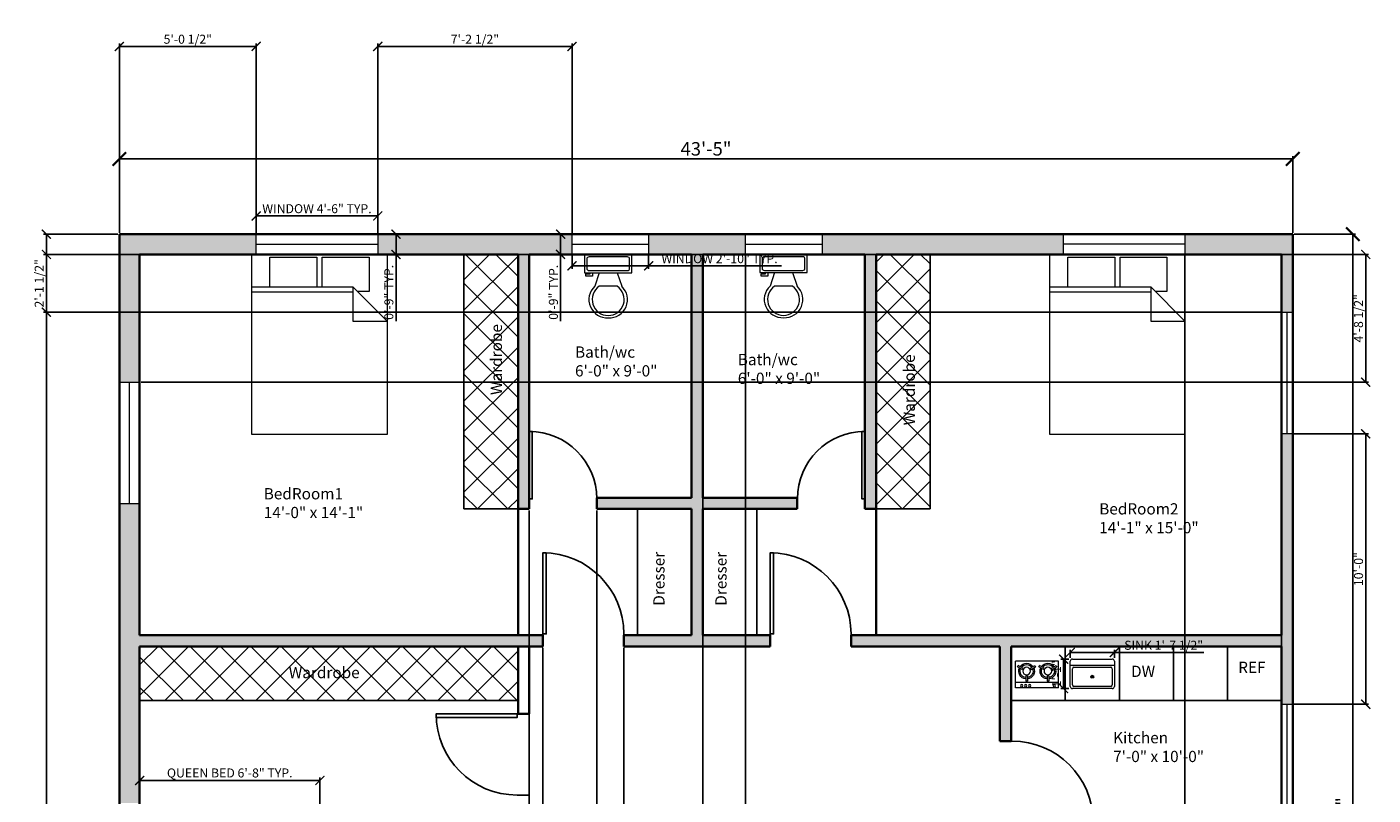
# Model space of a CAD drawing. Units: inches. Extents: x -43 to 8979, y -615 to 8149.
# Tile 3 of 5: x -43 to 555, y -235 to 106. Entities that reach past the tile are written whole.
import ezdxf

# ---------------------------------------------------------------- set-up
doc = ezdxf.new("R2010")
doc.units = ezdxf.units.IN
doc.header["$PDMODE"] = 35
doc.header["$PDSIZE"] = 5
for name, color, linetype, lineweight in [('A-ANNO-DIMS', 2, 'Continuous', 18), ('A-ANNO-TEXT', 7, 'Continuous', 18), ('A-AREA-IDEN', 7, 'Continuous', 25), ('A-DOOR', 4, 'Continuous', 25), ('A-EQPM', 8, 'Continuous', 18), ('A-FLOR-FIXT', 9, 'Continuous', 18), ('A-FURN', 9, 'Continuous', 18), ('A-GLAZ', 4, 'Continuous', 18), ('A-MILL', 30, 'Continuous', 25), ('A-MILL-PATT', 252, 'Continuous', 13), ('A-WALL', 7, 'Continuous', 35), ('A-WALL-PATT', 1, 'Continuous', 13)]:
    doc.layers.add(name, color=color, linetype=linetype, lineweight=lineweight)
doc.styles.get("Standard").update_dxf_attribs({"font": 'arial.ttf'})
doc.dimstyles.new('ISO-25', dxfattribs={"dimtxt": 4, "dimasz": 4, "dimexe": 1.25, "dimexo": 0.625, "dimtad": 1, "dimlunit": 3, "dimtxsty": 'Standard', "dimblk": 'ARCHTICK', "dimcen": 2.5, "dimadec": 0, "dimazin": 0, "dimtfac": 1, "dimtmove": 0, "dimatfit": 3, "dimfxl": 1, "dimarcsym": 0})

# ---------------------------------------------------------------- blocks, each defined once
blk = doc.blocks.new('*U3')
for p, q in [((0, 0), (0, -6)), ((40, 0), (40, -6))]:
    blk.add_line(p, q)
blk.add_lwpolyline([(0, 0), (0, 40), (1.75, 40), (1.75, 0)], close=True)
blk.add_arc((0, 0), 40, 0, 90)
blk = doc.blocks.new('Bed - Queen')
for p, q in [((0, -80.00003), (0, 0)), ((0, 0), (59.99999, 0)), ((59.99999, 0), (59.99999, -80.00003)), ((7.99999, -1.2), (28.79998, -1.2)), ((7.99999, -14.4), (7.99999, -1.2)), ((28.79998, -1.2), (28.79998, -14.4)), ((31.19999, -1.2), (51.99999, -1.2)), ((31.19999, -14.4), (31.19999, -1.2)), ((51.99999, -1.2), (51.99999, -16.4)), ((0, -14.4), (44.8, -14.4)), ((44.8, -16.8), (0, -16.8)), ((59.99999, -29.6), (44.8, -14.4)), ((44.8, -14.4), (44.8, -29.6)), ((51.99999, -16.4), (46.79936, -16.4)), ((44.8, -29.6), (59.99999, -29.6)), ((59.99999, -80.00003), (0, -80.00003))]:
    blk.add_line(p, q)
blk = doc.blocks.new('Sink-single - 30 in top')
blk.add_line((-15, -3.999996), (15, -3.999996))
for points in [[(-13.5, 0), (13.5, 0)], [(-15, -18.499996), (-15, -1.5)], [(-13.5, -17.499996), (-13.5, -6.499996)], [(-12.5, -5.499996), (12.5, -5.499996)], [(13.5, -6.499996), (13.5, -17.499996)], [(15, -1.5), (15, -18.499996)], [(13.5, -19.999996), (-13.5, -19.999996)], [(12.5, -18.499996), (-12.5, -18.499996)]]:
    blk.add_lwpolyline(points)
for radius in [1, 0.5]:
    blk.add_circle((0, -11.999996), radius)
for centre, radius, start, end in [((-13.5, -1.5), 1.5, 90, 180), ((-12.5, -6.499996), 1, 90, 180), ((12.5, -6.499996), 1, 0, 90), ((13.5, -1.5), 1.5, 0, 90), ((-12.5, -17.499996), 1, 180, 270), ((12.5, -17.499996), 1, 270, 0), ((-13.5, -18.499996), 1.5, 180, 270), ((13.5, -18.499996), 1.5, 270, 0)]:
    blk.add_arc(centre, radius, start, end)
blk = doc.blocks.new('*U7')
for p, q in [((9.5, -6), (9.5, -2)), ((-10, -8.5), (-8, -8.5)), ((-10, -9.5), (-10, -8.5)), ((-7, -9.5), (-10, -9.5)), ((-8, -8.5), (-8, -8)), ((-7, -8), (-7, -9.5)), ((-4, -8), (-6, -14)), ((4, -8), (6, -14)), ((4, -14), (-4, -14))]:
    blk.add_line(p, q)
blk.add_lwpolyline([(10.5, -8), (10.5, 0), (-10.5, 0), (-10.5, -8)], close=True)
for points in [[(-9.5, -2), (-9.5, -6)], [(8.5, -1), (-8.5, -1)], [(-8.5, -7), (8.5, -7)]]:
    blk.add_lwpolyline(points)
for centre, radius, start, end in [((-8.625, -1.875), 0.8839, 81.8699, 188.1301), ((8.625, -1.875), 0.8839, 351.8699, 98.1301), ((-8.625, -6.125), 0.8839, 171.869898, 278.1301), ((8.625, -6.125), 0.8839, 261.8699, 8.1301), ((-0.4772, -19.9188), 8.0953, 133.01722, 273.38), ((0.0374, -19.8731), 7.127, 124.50543, 269.7), ((-0.0373, -19.8731), 7.127, 270.3, 55.4946), ((0.4773, -19.9188), 8.0953, 266.62, 46.9828)]:
    blk.add_arc(centre, radius, start, end)
blk = doc.blocks.new('_ArchTick')
at = {"color": 0, "linetype": 'ByBlock', "const_width": 0.15}
blk.add_lwpolyline([(-0.5, -0.5), (0.5, 0.5)], dxfattribs=at)
blk = doc.blocks.new('*D12')
at = {"layer": 'A-ANNO-DIMS', "color": 0, "lineweight": -2, "transparency": 16777216}
for p, q in [((-1.95, 14.92), (-1.95, 48.94)), ((519.05, 14.92), (519.05, 48.94)), ((-1.95, 47.69), (519.05, 47.69))]:
    blk.add_line(p, q, dxfattribs=at)
at = {"layer": 'Defpoints', "color": 0, "transparency": 16777216}
for p in [(519.05, 47.69), (-1.95, 14.3), (519.05, 14.3)]:
    blk.add_point(p, dxfattribs=at)
at = {"layer": 'A-ANNO-DIMS', "color": 0, "lineweight": -2, "transparency": 16777216, "xscale": 6, "yscale": 6, "zscale": 6, "rotation": 180}
blk.add_blockref('_ArchTick', (-1.95, 47.69), dxfattribs=at)
at = {"layer": 'A-ANNO-DIMS', "color": 0, "lineweight": -2, "transparency": 16777216, "xscale": 6, "yscale": 6, "zscale": 6}
blk.add_blockref('_ArchTick', (519.05, 47.69), dxfattribs=at)
at = {"layer": 'A-ANNO-DIMS', "color": 0, "transparency": 16777216, "insert": (258.55, 51.38), "char_height": 6, "attachment_point": 5}
blk.add_mtext('43\'-5"', dxfattribs=at)
blk = doc.blocks.new('*D13')
at = {"layer": 'A-ANNO-DIMS', "color": 0, "lineweight": -2, "transparency": 16777216}
for p, q in [((519.68, 14.3), (546.94, 14.3)), ((545.69, 14.3), (545.69, -512.7)), ((519.68, -512.7), (546.94, -512.7))]:
    blk.add_line(p, q, dxfattribs=at)
at = {"layer": 'Defpoints', "color": 0, "transparency": 16777216}
for p in [(519.05, 14.3), (519.05, -512.7), (545.69, -512.7)]:
    blk.add_point(p, dxfattribs=at)
at = {"layer": 'A-ANNO-DIMS', "color": 0, "lineweight": -2, "transparency": 16777216, "xscale": 6, "yscale": 6, "zscale": 6}
for p, rotation in [((545.69, 14.3), 90), ((545.69, -512.7), 270)]:
    blk.add_blockref('_ArchTick', p, dxfattribs=dict(at, rotation=rotation))
at = {"layer": 'A-ANNO-DIMS', "color": 0, "transparency": 16777216, "insert": (541.99, -249.2), "char_height": 6, "attachment_point": 5, "rotation": 90}
blk.add_mtext('43\'-11"', dxfattribs=at)
blk = doc.blocks.new('WIN-54x9')
blk.add_line((4.5, 0), (4.5, 54))
blk.add_lwpolyline([(0, 0), (0, 54), (9, 54), (9, 0)], close=True)
blk = doc.blocks.new('WIN-34x9')
blk.add_line((4.5, 0), (4.5, 34))
blk.add_lwpolyline([(0, 0), (0, 34), (9, 34), (9, 0)], close=True)
blk = doc.blocks.new('WIN-54x5')
blk.add_line((2.5, 0), (2.5, 54))
blk.add_lwpolyline([(5, 54), (5, 0), (0, 0), (0, 54)], close=True)
blk = doc.blocks.new('COOKTOP-2-BURNER')
for p, q in [((19.04, 11.9), (0, 11.9)), ((0, 0), (0, 11.9)), ((0.88, 9.37), (1.24, 9.98)), ((2.94, 8.18), (0.88, 9.37)), ((3.3, 8.8), (1.24, 9.98)), ((2.94, 8.18), (3.3, 8.8)), ((6.55, 8.8), (8.6, 9.98)), ((6.55, 8.8), (6.9, 8.18)), ((6.9, 8.18), (8.96, 9.36)), ((8.6, 9.98), (8.96, 9.36)), ((10.35, 9.37), (10.7, 9.98)), ((12.4, 8.18), (10.35, 9.37)), ((12.76, 8.8), (10.7, 9.98)), ((12.4, 8.18), (12.76, 8.8)), ((16.01, 8.8), (18.06, 9.98)), ((16.01, 8.8), (16.36, 8.18)), ((16.36, 8.18), (18.42, 9.36)), ((18.06, 9.98), (18.42, 9.36)), ((19.04, 0), (19.04, 11.9)), ((19.04, 2.38), (0, 2.38)), ((19.04, 0), (0, 0)), ((4.56, 5.36), (4.56, 2.99)), ((5.28, 5.36), (4.56, 5.36)), ((5.28, 2.99), (4.56, 2.99)), ((5.28, 5.36), (5.28, 2.99)), ((14.02, 5.36), (14.02, 2.99)), ((14.74, 5.36), (14.02, 5.36)), ((14.74, 2.99), (14.02, 2.99)), ((14.74, 5.36), (14.74, 2.99))]:
    blk.add_line(p, q)
at = {"extrusion": (0, 0, -1)}
for centre, major_axis, start_param, end_param in [((4.92, 7.45), (0, 3.49), 3.2451, 5.134376), ((4.92, 7.45), (-2.04, 2.04), 4.051123, 5.898002), ((4.92, 7.45), (-0.01, 3.49), -0.942584, 0.946692), ((4.92, 7.45), (-2.04, 2.04), 6.145519, 7.992397), ((4.92, 7.45), (-1.2, 1.2), 2.356194490192311, 8.639379797371898), ((4.92, 7.45), (0, 3.49), 1.148752, 3.038029), ((4.92, 7.45), (2.04, 2.04), 0.385932, 2.23281), ((14.38, 7.45), (0, 3.49), 3.244173, 5.13345), ((14.38, 7.45), (2.04, 2.04), 2.480327, 4.327205), ((14.38, 7.45), (0, 3.49), -0.944011, 0.945266), ((14.38, 7.45), (-2.04, 2.04), 6.145519, 7.992397), ((14.38, 7.45), (-1.2, 1.2), 2.356194490192306, 8.639379797371893), ((14.38, 7.45), (0, 3.49), 1.14879, 3.038067), ((14.38, 7.45), (2.04, 2.04), 0.385932, 2.23281), ((2.71, 0.97), (-0.365, 0.365), 2.356194490192189, 8.639379797371776), ((4.5, 0.97), (-0.365, 0.365), 2.356194490192189, 8.639379797371776), ((6.25, 0.97), (-0.365, 0.365), 2.356194490192189, 8.639379797371776), ((17.3, 0.97), (-0.365, 0.365), 2.356194490192189, 8.639379797371776)]:
    blk.add_ellipse(centre, major_axis=major_axis, ratio=1, start_param=start_param, end_param=end_param, dxfattribs=at)
blk = doc.blocks.new('*D23')
at = {"layer": 'A-ANNO-DIMS', "color": 0, "lineweight": -2, "transparency": 16777216}
for p, q in [((7.05, -239.58), (7.05, -226.96)), ((87.05, -239.58), (87.05, -226.96)), ((87.05, -228.21), (7.05, -228.21))]:
    blk.add_line(p, q, dxfattribs=at)
at = {"layer": 'Defpoints', "color": 0, "transparency": 16777216}
for p in [(7.05, -228.21), (7.05, -240.21), (87.05, -240.21)]:
    blk.add_point(p, dxfattribs=at)
at = {"layer": 'A-ANNO-DIMS', "color": 0, "lineweight": -2, "transparency": 16777216, "xscale": 4, "yscale": 4, "zscale": 4, "rotation": 180}
blk.add_blockref('_ArchTick', (7.05, -228.21), dxfattribs=at)
at = {"layer": 'A-ANNO-DIMS', "color": 0, "lineweight": -2, "transparency": 16777216, "xscale": 4, "yscale": 4, "zscale": 4}
blk.add_blockref('_ArchTick', (87.05, -228.21), dxfattribs=at)
at = {"layer": 'A-ANNO-DIMS', "color": 0, "transparency": 16777216, "insert": (47.05, -225.39), "char_height": 4, "attachment_point": 5}
blk.add_mtext('QUEEN BED 6\'-8" TYP.', dxfattribs=at)
blk = doc.blocks.new('*D25')
at = {"layer": 'A-ANNO-DIMS', "color": 0, "lineweight": -2, "transparency": 16777216}
for p, q in [((58.78, 14.91), (58.78, 23.63)), ((58.78, 22.38), (112.78, 22.38)), ((112.78, 14.91), (112.78, 23.63))]:
    blk.add_line(p, q, dxfattribs=at)
at = {"layer": 'Defpoints', "color": 0, "transparency": 16777216}
for p in [(112.78, 22.38), (58.78, 14.28), (112.78, 14.28)]:
    blk.add_point(p, dxfattribs=at)
at = {"layer": 'A-ANNO-DIMS', "color": 0, "lineweight": -2, "transparency": 16777216, "xscale": 4, "yscale": 4, "zscale": 4, "rotation": 180}
blk.add_blockref('_ArchTick', (58.78, 22.38), dxfattribs=at)
at = {"layer": 'A-ANNO-DIMS', "color": 0, "lineweight": -2, "transparency": 16777216, "xscale": 4, "yscale": 4, "zscale": 4}
blk.add_blockref('_ArchTick', (112.78, 22.38), dxfattribs=at)
at = {"layer": 'A-ANNO-DIMS', "color": 0, "transparency": 16777216, "insert": (85.78, 25.07), "char_height": 4, "attachment_point": 5}
blk.add_mtext('WINDOW 4\'-6" TYP.', dxfattribs=at)
blk = doc.blocks.new('*D26')
at = {"layer": 'A-ANNO-DIMS', "color": 0, "lineweight": -2, "transparency": 16777216}
for p, q in [((113.41, 14.28), (122.13, 14.28)), ((120.88, 14.28), (120.88, 5.28)), ((113.41, 5.28), (122.13, 5.28)), ((120.88, 5.28), (120.88, -24.35))]:
    blk.add_line(p, q, dxfattribs=at)
at = {"layer": 'Defpoints', "color": 0, "transparency": 16777216}
for p in [(112.78, 14.28), (112.78, 5.28), (120.88, 5.28)]:
    blk.add_point(p, dxfattribs=at)
at = {"layer": 'A-ANNO-DIMS', "color": 0, "lineweight": -2, "transparency": 16777216, "xscale": 4, "yscale": 4, "zscale": 4}
for p, rotation in [((120.88, 14.28), 90), ((120.88, 5.28), 270)]:
    blk.add_blockref('_ArchTick', p, dxfattribs=dict(at, rotation=rotation))
at = {"layer": 'A-ANNO-DIMS', "color": 0, "transparency": 16777216, "insert": (118.22, -11.54), "char_height": 4, "attachment_point": 5, "rotation": 90}
blk.add_mtext('0\'-9" TYP.', dxfattribs=at)
blk = doc.blocks.new('*D29')
at = {"layer": 'A-ANNO-DIMS', "color": 0, "lineweight": -2, "transparency": 16777216}
for p, q in [((199.05, 4.67), (199.05, -1.05)), ((199.05, 0.2), (233.05, 0.2)), ((233.05, 4.67), (233.05, -1.05)), ((233.05, 0.2), (292.03, 0.2))]:
    blk.add_line(p, q, dxfattribs=at)
at = {"layer": 'Defpoints', "color": 0, "transparency": 16777216}
for p in [(199.05, 5.3), (233.05, 5.3), (233.05, 0.2)]:
    blk.add_point(p, dxfattribs=at)
at = {"layer": 'A-ANNO-DIMS', "color": 0, "lineweight": -2, "transparency": 16777216, "xscale": 4, "yscale": 4, "zscale": 4, "rotation": 180}
blk.add_blockref('_ArchTick', (199.05, 0.2), dxfattribs=at)
at = {"layer": 'A-ANNO-DIMS', "color": 0, "lineweight": -2, "transparency": 16777216, "xscale": 4, "yscale": 4, "zscale": 4}
blk.add_blockref('_ArchTick', (233.05, 0.2), dxfattribs=at)
at = {"layer": 'A-ANNO-DIMS', "color": 0, "transparency": 16777216, "insert": (264.54, 2.89), "char_height": 4, "attachment_point": 5}
blk.add_mtext('WINDOW 2\'-10" TYP.', dxfattribs=at)
blk = doc.blocks.new('*D30')
at = {"layer": 'A-ANNO-DIMS', "color": 0, "lineweight": -2, "transparency": 16777216}
for p, q in [((198.43, 14.3), (192.7, 14.3)), ((193.95, 14.3), (193.95, 5.3)), ((198.43, 5.3), (192.7, 5.3)), ((193.95, 5.3), (193.95, -24.33))]:
    blk.add_line(p, q, dxfattribs=at)
at = {"layer": 'Defpoints', "color": 0, "transparency": 16777216}
for p in [(199.05, 14.3), (193.95, 5.3), (199.05, 5.3)]:
    blk.add_point(p, dxfattribs=at)
at = {"layer": 'A-ANNO-DIMS', "color": 0, "lineweight": -2, "transparency": 16777216, "xscale": 4, "yscale": 4, "zscale": 4}
for p, rotation in [((193.95, 14.3), 90), ((193.95, 5.3), 270)]:
    blk.add_blockref('_ArchTick', p, dxfattribs=dict(at, rotation=rotation))
at = {"layer": 'A-ANNO-DIMS', "color": 0, "transparency": 16777216, "insert": (191.29, -11.52), "char_height": 4, "attachment_point": 5, "rotation": 90}
blk.add_mtext('0\'-9" TYP.', dxfattribs=at)
blk = doc.blocks.new('*D33')
at = {"layer": 'A-ANNO-DIMS', "color": 0, "lineweight": -2, "transparency": 16777216}
for p, q in [((420.24, -173.72), (420.24, -170.15)), ((420.24, -171.4), (439.85, -171.4)), ((439.85, -173.72), (439.85, -170.15)), ((439.85, -171.4), (479.63, -171.4))]:
    blk.add_line(p, q, dxfattribs=at)
at = {"layer": 'Defpoints', "color": 0, "transparency": 16777216}
for p in [(439.85, -171.4), (420.24, -174.34), (439.85, -174.34)]:
    blk.add_point(p, dxfattribs=at)
at = {"layer": 'A-ANNO-DIMS', "color": 0, "lineweight": -2, "transparency": 16777216, "xscale": 4, "yscale": 4, "zscale": 4, "rotation": 180}
blk.add_blockref('_ArchTick', (420.24, -171.4), dxfattribs=at)
at = {"layer": 'A-ANNO-DIMS', "color": 0, "lineweight": -2, "transparency": 16777216, "xscale": 4, "yscale": 4, "zscale": 4}
blk.add_blockref('_ArchTick', (439.85, -171.4), dxfattribs=at)
at = {"layer": 'A-ANNO-DIMS', "color": 0, "transparency": 16777216, "insert": (461.74, -168.71), "char_height": 4, "attachment_point": 5}
blk.add_mtext('SINK 1\'-7 1/2"', dxfattribs=at)
blk = doc.blocks.new('*D34')
at = {"layer": 'A-ANNO-DIMS', "color": 0, "lineweight": -2, "transparency": 16777216}
for p, q in [((419.62, -174.34), (416.05, -174.34)), ((417.3, -187.41), (417.3, -174.34)), ((419.62, -187.41), (416.05, -187.41))]:
    blk.add_line(p, q, dxfattribs=at)
at = {"layer": 'Defpoints', "color": 0, "transparency": 16777216}
for p in [(417.3, -174.34), (420.24, -174.34), (420.24, -187.41)]:
    blk.add_point(p, dxfattribs=at)
at = {"layer": 'A-ANNO-DIMS', "color": 0, "lineweight": -2, "transparency": 16777216, "xscale": 4, "yscale": 4, "zscale": 4}
for p, rotation in [((417.3, -174.34), 90), ((417.3, -187.41), 270)]:
    blk.add_blockref('_ArchTick', p, dxfattribs=dict(at, rotation=rotation))
at = {"layer": 'A-ANNO-DIMS', "color": 0, "transparency": 16777216, "insert": (414.67, -180.88), "char_height": 4, "attachment_point": 5, "rotation": 90}
blk.add_mtext('1\'-1"', dxfattribs=at)
blk = doc.blocks.new('*D41')
at = {"layer": 'A-ANNO-DIMS', "color": 0, "lineweight": -2, "transparency": 16777216}
for p, q in [((-1.95, 14.92), (-1.95, 98.86)), ((-1.95, 97.61), (58.78, 97.61)), ((58.78, 14.91), (58.78, 98.86))]:
    blk.add_line(p, q, dxfattribs=at)
at = {"layer": 'Defpoints', "color": 0, "transparency": 16777216}
for p in [(58.78, 97.61), (-1.95, 14.3), (58.78, 14.28)]:
    blk.add_point(p, dxfattribs=at)
at = {"layer": 'A-ANNO-DIMS', "color": 0, "lineweight": -2, "transparency": 16777216, "xscale": 4, "yscale": 4, "zscale": 4, "rotation": 180}
blk.add_blockref('_ArchTick', (-1.95, 97.61), dxfattribs=at)
at = {"layer": 'A-ANNO-DIMS', "color": 0, "lineweight": -2, "transparency": 16777216, "xscale": 4, "yscale": 4, "zscale": 4}
blk.add_blockref('_ArchTick', (58.78, 97.61), dxfattribs=at)
at = {"layer": 'A-ANNO-DIMS', "color": 0, "transparency": 16777216, "insert": (28.42, 100.3), "char_height": 4, "attachment_point": 5}
blk.add_mtext('5\'-0 1/2"', dxfattribs=at)
blk = doc.blocks.new('*D42')
at = {"layer": 'A-ANNO-DIMS', "color": 0, "lineweight": -2, "transparency": 16777216}
for p, q in [((112.78, 14.91), (112.78, 98.86)), ((112.78, 97.61), (199.05, 97.61)), ((199.05, 14.92), (199.05, 98.86))]:
    blk.add_line(p, q, dxfattribs=at)
at = {"layer": 'Defpoints', "color": 0, "transparency": 16777216}
for p in [(199.05, 97.61), (112.78, 14.28), (199.05, 14.3)]:
    blk.add_point(p, dxfattribs=at)
at = {"layer": 'A-ANNO-DIMS', "color": 0, "lineweight": -2, "transparency": 16777216, "xscale": 4, "yscale": 4, "zscale": 4, "rotation": 180}
blk.add_blockref('_ArchTick', (112.78, 97.61), dxfattribs=at)
at = {"layer": 'A-ANNO-DIMS', "color": 0, "lineweight": -2, "transparency": 16777216, "xscale": 4, "yscale": 4, "zscale": 4}
blk.add_blockref('_ArchTick', (199.05, 97.61), dxfattribs=at)
at = {"layer": 'A-ANNO-DIMS', "color": 0, "transparency": 16777216, "insert": (155.92, 100.3), "char_height": 4, "attachment_point": 5}
blk.add_mtext('7\'-2 1/2"', dxfattribs=at)
blk = doc.blocks.new('*D43')
at = {"layer": 'A-ANNO-DIMS', "color": 0, "lineweight": -2, "transparency": 16777216}
for p, q in [((257.05, 4.67), (257.05, -612.69)), ((276.05, 4.67), (276.05, -612.69)), ((257.05, -611.44), (276.05, -611.44))]:
    blk.add_line(p, q, dxfattribs=at)
at = {"layer": 'Defpoints', "color": 0, "transparency": 16777216}
for p in [(257.05, 5.3), (276.05, 5.3), (276.05, -611.44)]:
    blk.add_point(p, dxfattribs=at)
at = {"layer": 'A-ANNO-DIMS', "color": 0, "lineweight": -2, "transparency": 16777216, "xscale": 4, "yscale": 4, "zscale": 4, "rotation": 180}
blk.add_blockref('_ArchTick', (257.05, -611.44), dxfattribs=at)
at = {"layer": 'A-ANNO-DIMS', "color": 0, "lineweight": -2, "transparency": 16777216, "xscale": 4, "yscale": 4, "zscale": 4}
blk.add_blockref('_ArchTick', (276.05, -611.44), dxfattribs=at)
at = {"layer": 'A-ANNO-DIMS', "color": 0, "transparency": 16777216, "insert": (266.55, -608.8), "char_height": 4, "attachment_point": 5}
blk.add_mtext('1\'-7"', dxfattribs=at)
blk = doc.blocks.new('*D44')
at = {"layer": 'A-ANNO-DIMS', "color": 0, "lineweight": -2, "transparency": 16777216}
for p, q in [((471.21, 4.67), (471.21, -612.69)), ((514.05, 4.67), (514.05, -612.69)), ((471.21, -611.44), (514.05, -611.44))]:
    blk.add_line(p, q, dxfattribs=at)
at = {"layer": 'Defpoints', "color": 0, "transparency": 16777216}
for p in [(471.21, 5.3), (514.05, 5.3), (514.05, -611.44)]:
    blk.add_point(p, dxfattribs=at)
at = {"layer": 'A-ANNO-DIMS', "color": 0, "lineweight": -2, "transparency": 16777216, "xscale": 4, "yscale": 4, "zscale": 4, "rotation": 180}
blk.add_blockref('_ArchTick', (471.21, -611.44), dxfattribs=at)
at = {"layer": 'A-ANNO-DIMS', "color": 0, "lineweight": -2, "transparency": 16777216, "xscale": 4, "yscale": 4, "zscale": 4}
blk.add_blockref('_ArchTick', (514.05, -611.44), dxfattribs=at)
at = {"layer": 'A-ANNO-DIMS', "color": 0, "transparency": 16777216, "insert": (492.63, -608.77), "char_height": 4, "attachment_point": 5}
blk.add_mtext('3\'-7"', dxfattribs=at)
blk = doc.blocks.new('*D45')
at = {"layer": 'A-ANNO-DIMS', "color": 0, "lineweight": -2, "transparency": 16777216}
for p, q in [((7.68, 5.3), (552.7, 5.3)), ((551.45, 5.3), (551.45, -51.44)), ((7.68, -51.44), (552.7, -51.44))]:
    blk.add_line(p, q, dxfattribs=at)
at = {"layer": 'Defpoints', "color": 0, "transparency": 16777216}
for p in [(7.05, 5.3), (7.05, -51.44), (551.45, -51.44)]:
    blk.add_point(p, dxfattribs=at)
at = {"layer": 'A-ANNO-DIMS', "color": 0, "lineweight": -2, "transparency": 16777216, "xscale": 4, "yscale": 4, "zscale": 4}
for p, rotation in [((551.45, 5.3), 90), ((551.45, -51.44), 270)]:
    blk.add_blockref('_ArchTick', p, dxfattribs=dict(at, rotation=rotation))
at = {"layer": 'A-ANNO-DIMS', "color": 0, "transparency": 16777216, "insert": (548.76, -23.07), "char_height": 4, "attachment_point": 5, "rotation": 90}
blk.add_mtext('4\'-8 1/2"', dxfattribs=at)
blk = doc.blocks.new('*D48')
at = {"layer": 'A-ANNO-DIMS', "color": 0, "lineweight": -2, "transparency": 16777216}
for p, q in [((513.43, 5.3), (-35.6, 5.3)), ((-34.35, 5.3), (-34.35, -20.37)), ((513.43, -20.37), (-35.6, -20.37))]:
    blk.add_line(p, q, dxfattribs=at)
at = {"layer": 'Defpoints', "color": 0, "transparency": 16777216}
for p in [(514.05, 5.3), (-34.35, -20.37), (514.05, -20.37)]:
    blk.add_point(p, dxfattribs=at)
at = {"layer": 'A-ANNO-DIMS', "color": 0, "lineweight": -2, "transparency": 16777216, "xscale": 4, "yscale": 4, "zscale": 4}
for p, rotation in [((-34.35, 5.3), 90), ((-34.35, -20.37), 270)]:
    blk.add_blockref('_ArchTick', p, dxfattribs=dict(at, rotation=rotation))
at = {"layer": 'A-ANNO-DIMS', "color": 0, "transparency": 16777216, "insert": (-37.04, -7.53), "char_height": 4, "attachment_point": 5, "rotation": 90}
blk.add_mtext('2\'-1 1/2"', dxfattribs=at)
blk = doc.blocks.new('*D49')
at = {"layer": 'A-ANNO-DIMS', "color": 0, "lineweight": -2, "transparency": 16777216}
for p, q in [((519.68, -74.37), (552.7, -74.37)), ((551.45, -74.37), (551.45, -194.4)), ((519.68, -194.4), (552.7, -194.4))]:
    blk.add_line(p, q, dxfattribs=at)
at = {"layer": 'Defpoints', "color": 0, "transparency": 16777216}
for p in [(519.05, -74.37), (519.05, -194.4), (551.45, -194.4)]:
    blk.add_point(p, dxfattribs=at)
at = {"layer": 'A-ANNO-DIMS', "color": 0, "lineweight": -2, "transparency": 16777216, "xscale": 4, "yscale": 4, "zscale": 4}
for p, rotation in [((551.45, -74.37), 90), ((551.45, -194.4), 270)]:
    blk.add_blockref('_ArchTick', p, dxfattribs=dict(at, rotation=rotation))
at = {"layer": 'A-ANNO-DIMS', "color": 0, "transparency": 16777216, "insert": (548.79, -134.38), "char_height": 4, "attachment_point": 5, "rotation": 90}
blk.add_mtext('10\'-0"', dxfattribs=at)
blk = doc.blocks.new('*D53')
at = {"layer": 'A-ANNO-DIMS', "color": 0, "lineweight": -2, "transparency": 16777216}
for p, q in [((-2.57, 14.3), (-35.6, 14.3)), ((-34.35, 14.3), (-34.35, -578.78)), ((259.43, -578.78), (-35.6, -578.78))]:
    blk.add_line(p, q, dxfattribs=at)
at = {"layer": 'Defpoints', "color": 0, "transparency": 16777216}
for p in [(-1.95, 14.3), (-34.35, -578.78), (260.05, -578.78)]:
    blk.add_point(p, dxfattribs=at)
at = {"layer": 'A-ANNO-DIMS', "color": 0, "lineweight": -2, "transparency": 16777216, "xscale": 4, "yscale": 4, "zscale": 4}
for p, rotation in [((-34.35, 14.3), 90), ((-34.35, -578.78), 270)]:
    blk.add_blockref('_ArchTick', p, dxfattribs=dict(at, rotation=rotation))
at = {"layer": 'A-ANNO-DIMS', "color": 0, "transparency": 16777216, "insert": (-37.01, -282.24), "char_height": 4, "attachment_point": 5, "rotation": 90}
blk.add_mtext('49\'-5"', dxfattribs=at)
blk = doc.blocks.new('*D54')
at = {"layer": 'A-ANNO-DIMS', "color": 0, "lineweight": -2, "transparency": 16777216}
for p, q in [((180.05, -108.33), (180.05, -612.69)), ((210.05, -108.33), (210.05, -612.69)), ((180.05, -611.44), (210.05, -611.44))]:
    blk.add_line(p, q, dxfattribs=at)
at = {"layer": 'Defpoints', "color": 0, "transparency": 16777216}
for p in [(180.05, -107.7), (210.05, -107.7), (210.05, -611.44)]:
    blk.add_point(p, dxfattribs=at)
at = {"layer": 'A-ANNO-DIMS', "color": 0, "lineweight": -2, "transparency": 16777216, "xscale": 4, "yscale": 4, "zscale": 4, "rotation": 180}
blk.add_blockref('_ArchTick', (180.05, -611.44), dxfattribs=at)
at = {"layer": 'A-ANNO-DIMS', "color": 0, "lineweight": -2, "transparency": 16777216, "xscale": 4, "yscale": 4, "zscale": 4}
blk.add_blockref('_ArchTick', (210.05, -611.44), dxfattribs=at)
at = {"layer": 'A-ANNO-DIMS', "color": 0, "transparency": 16777216, "insert": (195.05, -608.77), "char_height": 4, "attachment_point": 5}
blk.add_mtext('2\'-6"', dxfattribs=at)
blk = doc.blocks.new('*D55')
at = {"layer": 'A-ANNO-DIMS', "color": 0, "lineweight": -2, "transparency": 16777216}
for p, q in [((186.05, -169.33), (186.05, -612.69)), ((222.05, -169.33), (222.05, -612.69)), ((186.05, -611.44), (222.05, -611.44))]:
    blk.add_line(p, q, dxfattribs=at)
at = {"layer": 'Defpoints', "color": 0, "transparency": 16777216}
for p in [(186.05, -168.7), (222.05, -168.7), (222.05, -611.44)]:
    blk.add_point(p, dxfattribs=at)
at = {"layer": 'A-ANNO-DIMS', "color": 0, "lineweight": -2, "transparency": 16777216, "xscale": 4, "yscale": 4, "zscale": 4, "rotation": 180}
blk.add_blockref('_ArchTick', (186.05, -611.44), dxfattribs=at)
at = {"layer": 'A-ANNO-DIMS', "color": 0, "lineweight": -2, "transparency": 16777216, "xscale": 4, "yscale": 4, "zscale": 4}
blk.add_blockref('_ArchTick', (222.05, -611.44), dxfattribs=at)
at = {"layer": 'A-ANNO-DIMS', "color": 0, "transparency": 16777216, "insert": (204.05, -608.77), "char_height": 4, "attachment_point": 5}
blk.add_mtext('3\'-0"', dxfattribs=at)

msp = doc.modelspace()

# ---------------------------------------------------------------- hatches: boundary and pattern name
at = {"layer": 'A-MILL-PATT'}
h = msp.add_hatch(dxfattribs=at)
h.set_pattern_fill('ANSI37', color=256, scale=3)
h.set_pattern_definition([(45, (-529.924, 6e-14), (-6.73519, 6.73519), []), (135, (-529.924, 6e-14), (-6.73519, -6.73519), [])])
h.paths.add_polyline_path([(175.054, -168.703), (7.054, -168.703), (7.054, -192.703), (175.054, -192.703)])
h.paths.add_polyline_path([(175.054, 5.297), (151.054, 5.297), (151.054, -107.703), (175.054, -107.703)])
h.paths.add_polyline_path([(358.054, 5.297), (334.054, 5.297), (334.054, -107.703), (358.054, -107.703)])
h.paths.add_polyline_path([(514.054, -346.703), (444.16, -346.703), (444.16, -370.703), (514.054, -370.703)])
at = {"layer": 'A-WALL-PATT'}
h = msp.add_hatch(color=256, dxfattribs=at)
h.dxf.hatch_style = 1
h.paths.add_polyline_path([(7.054, 5.297), (58.783, 5.297), (58.783, 14.297), (-1.946, 14.297), (-1.946, -51.444), (7.054, -51.444)])
h.paths.add_polyline_path([(7.054, -105.444), (-1.946, -105.444), (-1.946, -238.206), (7.054, -238.206), (7.054, -168.703), (175.054, -168.703), (180.054, -168.703), (186.046, -168.703), (186.046, -163.703), (175.054, -163.703), (7.054, -163.703)])
h.paths.add_polyline_path([(199.054, 14.297), (112.783, 14.297), (112.783, 5.297), (116.889, 5.297), (175.054, 5.297), (175.054, -107.703), (180.054, -107.703), (180.054, -103.21), (180.054, -73.263), (180.054, 5.297), (199.054, 5.297)])
h.paths.add_polyline_path([(276.054, 14.297), (233.054, 14.297), (233.054, 5.297), (252.054, 5.297), (252.054, -102.703), (210.054, -102.703), (210.054, -107.703), (252.054, -107.703), (252.054, -163.703), (222.054, -163.703), (222.054, -168.703), (286.948, -168.703), (286.948, -163.703), (257.054, -163.703), (257.054, -107.703), (299.054, -107.703), (299.054, -102.703), (257.054, -102.703), (257.054, 5.297), (276.054, 5.297)])
h.paths.add_polyline_path([(417.209, 14.297), (310.054, 14.297), (310.054, 5.297), (329.054, 5.297), (329.054, -107.703), (334.054, -107.703), (334.054, 5.297), (417.209, 5.297)])
h.paths.add_polyline_path([(519.054, 14.297), (471.209, 14.297), (471.209, 5.297), (514.054, 5.297), (514.054, -20.367), (519.054, -20.367)])
h.paths.add_polyline_path([(519.054, -74.367), (514.054, -74.367), (514.054, -163.703), (323.054, -163.703), (323.054, -168.703), (329.054, -168.703), (334.054, -168.703), (389.054, -168.703), (389.054, -210.703), (394.054, -210.703), (394.054, -168.703), (514.054, -168.703), (514.054, -194.4), (519.054, -194.4)])
h.paths.add_polyline_path([(519.054, -248.4), (514.054, -248.4), (514.054, -252.703), (394.054, -252.703), (394.054, -246.703), (389.054, -246.703), (389.054, -263.703), (394.054, -263.703), (394.054, -257.703), (514.054, -257.703), (514.054, -264.224), (519.054, -264.224)])

# ---------------------------------------------------------------- linework, layer by layer
at = {"layer": 'A-MILL'}
for p, q in [((151.054, 5.297), (151.054, -107.703)), ((358.054, -107.703), (358.054, 5.297)), ((175.054, -107.703), (151.054, -107.703)), ((228.054, -163.703), (228.054, -107.703)), ((281.054, -163.703), (281.054, -107.703)), ((334.054, -107.703), (358.054, -107.703)), ((418.054, -192.703), (418.054, -168.703)), ((442.088, -192.703), (442.088, -168.703)), ((466.088, -192.703), (466.088, -168.703)), ((490.088, -192.703), (490.088, -168.703)), ((7.054, -192.703), (175.054, -192.703)), ((394.054, -192.703), (514.054, -192.703))]:
    msp.add_line(p, q, dxfattribs=at)
at = {"layer": 'A-WALL'}
for p, q in [((-1.946, 14.297), (519.054, 14.297)), ((-1.946, -345.703), (-1.946, 14.297)), ((519.054, 14.297), (519.054, -512.703)), ((7.054, 5.297), (175.054, 5.297)), ((7.054, -163.703), (7.054, 5.297)), ((175.054, -107.703), (175.054, 5.297)), ((180.054, 5.297), (252.054, 5.297)), ((180.054, -107.703), (180.054, 5.297)), ((252.054, -102.703), (252.054, 5.297)), ((257.054, 5.297), (329.054, 5.297)), ((257.054, -102.703), (257.054, 5.297)), ((329.054, -107.703), (329.054, 5.297)), ((334.054, 5.297), (514.054, 5.297)), ((334.054, -107.703), (334.054, 5.297)), ((514.054, 5.297), (514.054, -163.703)), ((210.054, -102.703), (252.054, -102.703)), ((210.054, -107.703), (210.054, -102.703)), ((257.054, -102.703), (299.054, -102.703)), ((299.054, -107.703), (299.054, -102.703)), ((180.054, -107.703), (175.054, -107.703)), ((175.054, -107.703), (175.054, -163.703)), ((210.054, -107.703), (252.054, -107.703)), ((252.054, -163.703), (252.054, -107.703)), ((257.054, -107.703), (299.054, -107.703)), ((257.054, -163.703), (257.054, -107.703)), ((329.054, -107.703), (334.054, -107.703)), ((334.054, -107.703), (334.054, -163.703)), ((7.054, -163.703), (175.054, -163.703)), ((175.054, -163.703), (186.054, -163.703)), ((186.054, -168.703), (186.054, -163.703)), ((222.054, -168.703), (222.054, -163.703)), ((222.054, -163.703), (252.054, -163.703)), ((257.054, -163.703), (287.054, -163.703)), ((287.054, -163.703), (287.054, -168.703)), ((323.054, -163.703), (323.054, -168.703)), ((323.054, -163.703), (514.054, -163.703)), ((7.054, -168.703), (175.054, -168.703)), ((7.054, -336.703), (7.054, -168.703)), ((175.054, -168.703), (180.054, -168.703)), ((175.054, -198.703), (175.054, -168.703)), ((180.054, -168.703), (186.054, -168.703)), ((180.054, -198.703), (180.054, -168.703)), ((222.054, -168.703), (287.054, -168.703)), ((323.054, -168.703), (329.054, -168.703)), ((329.054, -168.703), (334.054, -168.703)), ((334.054, -168.703), (389.054, -168.703)), ((389.054, -168.703), (389.054, -210.703)), ((394.054, -168.703), (394.054, -210.703)), ((394.054, -168.703), (514.054, -168.703)), ((514.054, -168.703), (514.054, -252.703)), ((175.054, -198.703), (180.054, -198.703)), ((394.054, -210.703), (389.054, -210.703))]:
    msp.add_line(p, q, dxfattribs=at)

# ---------------------------------------------------------------- block references
at = {"layer": 'A-DOOR'}
for p, xscale, yscale, zscale in [((180.054, -103.21), 0.7486801686032757, 0.7486801686032757, 0.7486801686032757), ((329.054, -103.21), -0.7486801686032757, 0.7486801686032757, 0.7486801686032757), ((186.046, -163.16), 0.8992725759508509, 0.8992725759508509, 0.8992725759508509), ((286.948, -163.16), 0.8992725759508509, 0.8992725759508509, 0.8992725759508509)]:
    msp.add_blockref('*U3', p, dxfattribs=dict(at, xscale=xscale, yscale=yscale, zscale=zscale))
at = {"layer": 'A-DOOR', "xscale": -0.8992725759508509, "yscale": 0.8992725759508509, "zscale": 0.8992725759508509}
for p, rotation in [((174.659, -198.703), 90), ((394.45, -246.703), 270)]:
    msp.add_blockref('*U3', p, dxfattribs=dict(at, rotation=rotation))
at = {"layer": 'A-EQPM'}
msp.add_blockref('COOKTOP-2-BURNER', (395.944, -187.109), dxfattribs=at)
at = {"layer": 'A-FLOR-FIXT'}
for p in [(215.107, 5.16), (292.961, 5.211)]:
    msp.add_blockref('*U7', p, dxfattribs=at)
at = {"layer": 'A-FLOR-FIXT', "xscale": 0.6535598392555352, "yscale": 0.6535598392555352, "zscale": 0.6535598392555352}
msp.add_blockref('Sink-single - 30 in top', (430.047, -174.344), dxfattribs=at)
at = {"layer": 'A-FURN'}
for p in [(56.889, 5.297), (411.209, 5.297)]:
    msp.add_blockref('Bed - Queen', p, dxfattribs=at)
at = {"layer": 'A-GLAZ'}
for name, p, rotation in [('WIN-54x9', (58.783, 14.281), 270), ('WIN-34x9', (199.055, 14.298), 270.0000000000001), ('WIN-34x9', (276.055, 14.298), 270), ('WIN-54x9', (471.209, 5.297), 90)]:
    msp.add_blockref(name, p, dxfattribs=dict(at, rotation=rotation))
for name, p in [('WIN-54x5', (514.054, -74.367)), ('WIN-54x9', (-1.946, -105.444)), ('WIN-54x5', (514.054, -248.4))]:
    msp.add_blockref(name, p, dxfattribs=at)

# ---------------------------------------------------------------- texts
at = {"layer": 'A-ANNO-TEXT', "char_height": 5, "attachment_point": 1, "rotation": 90}
for s, width, insert in [('Wardrobe', 68.19541, (162.928, -57.105)), ('Wardrobe', 68.19541, (346.256, -70.539)), ('Dresser', 92.19772, (235.119, -150.645)), ('Dresser', 92.19772, (262.656, -150.645))]:
    msp.add_mtext_dynamic_manual_height_columns(s, width=width, gutter_width=12.5, heights=[0], dxfattribs=dict(at, insert=insert))
at = {"layer": 'A-ANNO-TEXT', "char_height": 5, "attachment_point": 1}
for s, width, insert in [('Wardrobe', 68.19541, (73.266, -177.811)), ('DW', 16.00427, (447.267, -177.266)), ('REF', 17.27895, (494.848, -175.49))]:
    msp.add_mtext_dynamic_manual_height_columns(s, width=width, gutter_width=12.5, heights=[0], dxfattribs=dict(at, insert=insert))
at = {"layer": 'A-AREA-IDEN', "char_height": 5, "attachment_point": 1}
for s, width, insert in [('Bath/wc\\P6\'-0" x 9\'-0"', 52.09042, (200.372, -35.551)), ('Bath/wc\\P6\'-0" x 9\'-0"', 52.09042, (272.648, -38.866)), ('BedRoom1\\P14\'-0" x 14\'-1"', 101.99671, (62.156, -98.436)), ('BedRoom2\\P14\'-1" x 15\'-0"', 101.99671, (433.124, -105.15)), ('Kitchen\\P7\'-0" x 10\'-0"', 76.04775, (439.299, -206.715))]:
    msp.add_mtext_dynamic_manual_height_columns(s, width=width, gutter_width=12.5, heights=[0], dxfattribs=dict(at, insert=insert))

# ---------------------------------------------------------------- dimensions: what is measured, and where the dimension line sits
at = {"layer": 'A-ANNO-DIMS'}
for base, p1, p2, override, picture, middle in [((58.783, 97.611), (-1.946, 14.297), (58.783, 14.28), {"dimdec": 1, "dimlfac": 1, "dimrnd": 0, "dimzin": 1, "dimdsep": 46, "dimlunit": 4, "dimfrac": 2}, '*D41', (28.419, 100.304)), ((199.054, 97.611), (112.783, 14.28), (199.054, 14.297), {"dimdec": 1, "dimlfac": 1, "dimrnd": 0, "dimzin": 1, "dimdsep": 46, "dimlunit": 4, "dimfrac": 2}, '*D42', (155.919, 100.304)), ((519.054, 47.69), (-1.946, 14.297), (519.054, 14.297), {"dimtxt": 6, "dimasz": 6, "dimclrd": 0, "dimclre": 0, "dimclrt": 0}, '*D12', (258.554, 51.381)), ((276.054, -611.437), (257.054, 5.297), (276.054, 5.297), {"dimdec": 1, "dimlfac": 1, "dimrnd": 0, "dimzin": 1, "dimdsep": 46, "dimlunit": 4, "dimfrac": 2}, '*D43', (266.554, -608.804)), ((514.054, -611.437), (471.209, 5.297), (514.054, 5.297), {"dimdec": 1, "dimlfac": 1, "dimrnd": 0, "dimzin": 1, "dimdsep": 46, "dimlunit": 4, "dimfrac": 2}, '*D44', (492.632, -608.769)), ((210.054, -611.437), (180.054, -107.703), (210.054, -107.703), {"dimdec": 1, "dimlfac": 1, "dimrnd": 0, "dimzin": 1, "dimdsep": 46, "dimlunit": 4, "dimfrac": 2}, '*D54', (195.054, -608.77)), ((222.054, -611.437), (186.054, -168.703), (222.054, -168.703), {"dimdec": 1, "dimlfac": 1, "dimrnd": 0, "dimzin": 1, "dimdsep": 46, "dimlunit": 4, "dimfrac": 2}, '*D55', (204.054, -608.769))]:
    dim = msp.add_linear_dim(base=base, p1=p1, p2=p2, dimstyle='ISO-25', override=override, dxfattribs=at)
    dim.commit()
    dim.dimension.update_dxf_attribs({"geometry": picture, "text_midpoint": middle})
for base, p1, p2, text, picture, middle in [((112.783, 22.38), (58.783, 14.28), (112.783, 14.28), 'WINDOW <> TYP.', '*D25', (85.783, 25.075)), ((439.851, -171.403), (420.244, -174.344), (439.851, -174.344), 'SINK <>', '*D33', (461.74, -168.709))]:
    dim = msp.add_linear_dim(base=base, p1=p1, p2=p2, text=text, dimstyle='ISO-25', override={"dimdec": 1, "dimlfac": 1, "dimrnd": 0, "dimzin": 1, "dimdsep": 46, "dimlunit": 4, "dimfrac": 2}, dxfattribs=at)
    dim.commit()
    dim.dimension.update_dxf_attribs({"geometry": picture, "text_midpoint": middle})
for base, p1, p2, override, picture, middle in [((-34.346, -578.784), (-1.946, 14.297), (260.054, -578.784), {"dimdec": 1, "dimlfac": 1, "dimrnd": 0, "dimzin": 1, "dimdsep": 46, "dimlunit": 4, "dimfrac": 2}, '*D53', (-37.013, -282.243)), ((545.685, -512.703), (519.054, 14.297), (519.054, -512.703), {"dimtxt": 6, "dimasz": 6, "dimclrd": 0, "dimclre": 0, "dimclrt": 0}, '*D13', (541.995, -249.203)), ((-34.346, -20.367), (514.054, 5.297), (514.054, -20.367), {"dimdec": 1, "dimlfac": 1, "dimrnd": 0, "dimzin": 1, "dimdsep": 46, "dimlunit": 4, "dimfrac": 2}, '*D48', (-37.039, -7.535)), ((551.454, -51.444), (7.054, 5.297), (7.054, -51.444), {"dimdec": 1, "dimlfac": 1, "dimrnd": 0, "dimzin": 1, "dimdsep": 46, "dimlunit": 4, "dimfrac": 2}, '*D45', (548.761, -23.073)), ((551.454, -194.4), (519.054, -74.367), (519.054, -194.4), {"dimdec": 1, "dimlfac": 1, "dimrnd": 0, "dimzin": 1, "dimdsep": 46, "dimlunit": 4, "dimfrac": 2}, '*D49', (548.787, -134.383)), ((417.303, -174.344), (420.244, -187.415), (420.244, -174.344), {"dimdec": 1, "dimlfac": 1, "dimrnd": 0, "dimzin": 1, "dimdsep": 46, "dimlunit": 4, "dimfrac": 2}, '*D34', (414.67, -180.879))]:
    dim = msp.add_linear_dim(base=base, p1=p1, p2=p2, angle=90, dimstyle='ISO-25', override=override, dxfattribs=at)
    dim.commit()
    dim.dimension.update_dxf_attribs({"geometry": picture, "text_midpoint": middle})
for base, p1, p2, angle, text, picture, middle in [((120.883, 5.28), (112.783, 14.28), (112.783, 5.28), 270, '<> TYP.', '*D26', (118.216, -11.536)), ((193.954, 5.297), (199.054, 14.297), (199.054, 5.297), 270, '<> TYP.', '*D30', (191.287, -11.519)), ((233.054, 0.197), (199.054, 5.297), (233.054, 5.297), 0, 'WINDOW <> TYP.', '*D29', (264.542, 2.892)), ((7.054, -228.206), (87.054, -240.206), (7.054, -240.206), 180, 'QUEEN BED <> TYP.', '*D23', (47.054, -225.39))]:
    dim = msp.add_linear_dim(base=base, p1=p1, p2=p2, angle=angle, text=text, dimstyle='ISO-25', override={"dimdec": 1, "dimlfac": 1, "dimrnd": 0, "dimzin": 1, "dimdsep": 46, "dimlunit": 4, "dimfrac": 2}, dxfattribs=at)
    dim.commit()
    dim.dimension.update_dxf_attribs({"geometry": picture, "text_midpoint": middle})

doc.saveas('drawing.dxf')
